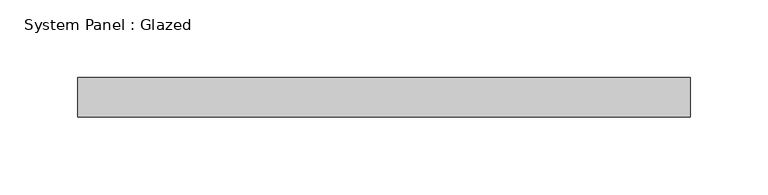
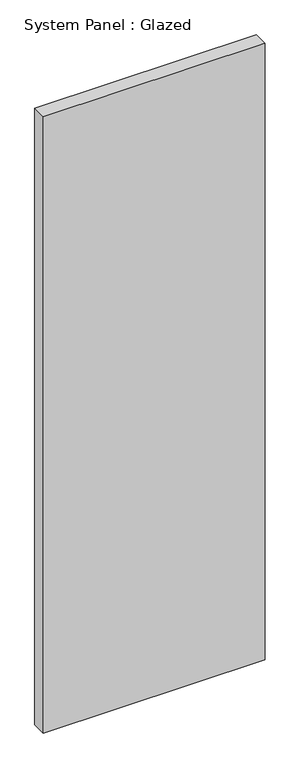
"""IFC4 building model written with IfcOpenShell, lengths in millimetres: plate geometry, System Panel : Glazed."""

from ifc_helpers import new_model, si_unit, origin, origin_with_axes, place, context, project, spatial, polyline, outline, extrude, source, transform, mapped, element, save


def system_panel_glazed_c3939aa2(model_context):
    return source(origin(), model_context, "Body", "SweptSolid", [
        extrude(outline(polyline([(196.85, 19.05), (-196.85, 19.05), (-196.85, 44.45), (196.85, 44.45), (196.85, 19.05)])), origin_with_axes(), (0.0, 0.0, 1.0), 1155.7),
    ])


if __name__ == "__main__":
    model = new_model("IFC4")
    model_context = context("Model", 3, world=origin())
    ifc_project = project(units=[si_unit("LENGTHUNIT", "METRE", prefix="MILLI")], contexts=[model_context])
    site = spatial("IfcSite", under=ifc_project)
    building = spatial("IfcBuilding", under=site)
    placement = place(None, origin())
    system_panel_glazed_shape = system_panel_glazed_c3939aa2(model_context)
    element("IfcPlate", 1, ObjectType="System Panel : Glazed", at=placement, inside=building, context=model_context, shape_type="MappedRepresentation", body=[
        mapped(system_panel_glazed_shape, transform((0.0, 0.0, 0.0), x_axis=(1.0, 0.0, 0.0), y_axis=(0.0, 1.0, 0.0), z_axis=(0.0, 0.0, 1.0))),
    ])
    save(model, "model.ifc")

# Revit data of these elements
# Type "System Panel : Glazed"
#   Construction Type Id = "GSP4R"
#   Analytic Construction = "1/8 in Pilkington single glazing"
#   Visual Light Transmittance = 0.9
#   Solar Heat Gain Coefficient = 0.86
#   Heat Transfer Coefficient (U) = 1.18115 BTU/(h·ft²·°F)
# Element 1 (IfcPlate, "System Panel : Glazed")
#   Materials on its faces: "Glass"
# Materials
#   "Glass": class "Glass", colour RGB 0 128 192, transparency 0.75, Description = "Soda Lime Glass", Cost = 0
